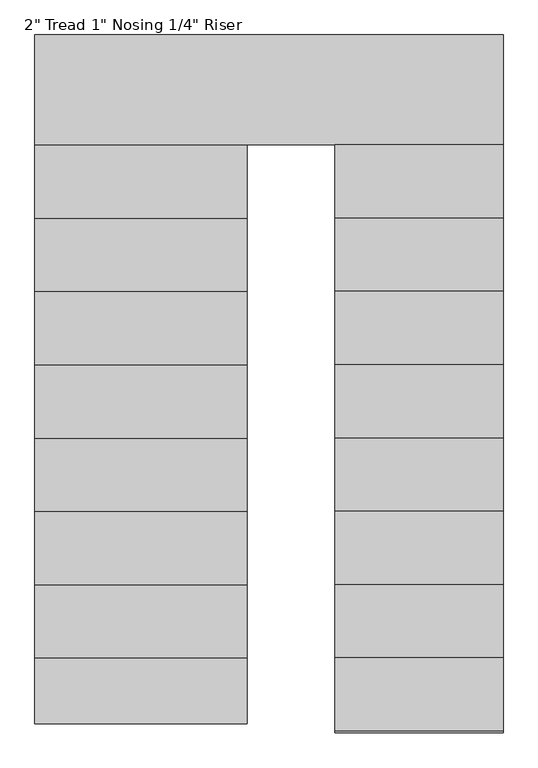
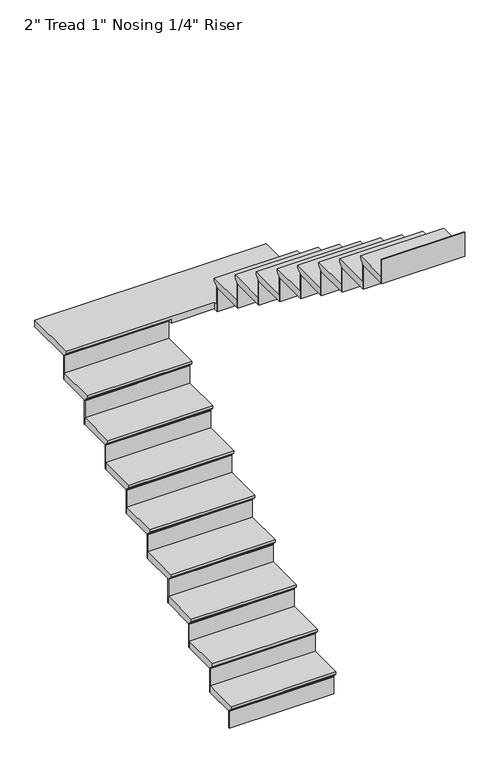
"""IFC4 building model written with IfcOpenShell, lengths in millimetres: stair flight geometry."""

from ifc_helpers import new_model, si_unit, origin, place, context, project, spatial, faceted_brep, source, transform, mapped, element, save


def stair_flight_4914edaa(model_context):
    return source(origin(), model_context, "Body", "Brep", [
        faceted_brep([(3394.0891134, -7650.9822004, 9759.95), (3394.0891134, -7650.9822004, 9779.0), (2657.4891134, -7650.9822004, 9779.0), (2657.4891134, -7650.9822004, 9759.95), (3394.0891134, -7625.5822004, 9734.55), (2657.4891134, -7625.5822004, 9734.55), (3394.0891134, -7396.9822004, 9779.0), (2657.4891134, -7396.9822004, 9779.0), (2657.4891134, -7625.5822004, 9728.2), (2657.4891134, -7396.9822004, 9728.2), (3394.0891134, -7396.9822004, 9728.2), (3394.0891134, -7625.5822004, 9728.2)], [[[0, 1, 2, 3]], [[4, 0, 3, 5]], [[2, 1, 6, 7]], [[8, 9, 10, 11]], [[2, 7, 9, 8, 5, 3]], [[8, 11, 4, 5]], [[6, 1, 0, 4, 11, 10]], [[7, 6, 10, 9]]]),
        faceted_brep([(3394.0891134, -7625.5822004, 9728.2), (3394.0891134, -7625.5822004, 9601.2), (3394.0891134, -7619.2322004, 9601.2), (3394.0891134, -7619.2322004, 9728.2), (2657.4891134, -7625.5822004, 9728.2), (2657.4891134, -7619.2322004, 9728.2), (2657.4891134, -7619.2322004, 9601.2), (2657.4891134, -7625.5822004, 9601.2)], [[[0, 1, 2, 3]], [[4, 5, 6, 7]], [[1, 0, 4, 7]], [[2, 1, 7, 6]], [[3, 2, 6, 5]], [[0, 3, 5, 4]]]),
        faceted_brep([(3394.0891134, -7396.9822004, 9906.0), (3394.0891134, -7396.9822004, 9728.2), (3394.0891134, -7390.6322004, 9728.2), (3394.0891134, -7390.6322004, 9906.0), (2657.4891134, -7396.9822004, 9906.0), (2657.4891134, -7390.6322004, 9906.0), (2657.4891134, -7390.6322004, 9728.2), (2657.4891134, -7396.9822004, 9728.2)], [[[0, 1, 2, 3]], [[4, 5, 6, 7]], [[1, 0, 4, 7]], [[2, 1, 7, 6]], [[3, 2, 6, 5]], [[0, 3, 5, 4]]]),
        faceted_brep([(2657.4891134, -7422.3822004, 9956.8), (3394.0891134, -7422.3822004, 9956.8), (3394.0891134, -7142.9822004, 9956.8), (2657.4891134, -7142.9822004, 9956.8), (2657.4891134, -7396.9822004, 9906.0), (2657.4891134, -7142.9822004, 9906.0), (3394.0891134, -7142.9822004, 9906.0), (3394.0891134, -7396.9822004, 9906.0), (2657.4891134, -7396.9822004, 9912.35), (2657.4891134, -7422.3822004, 9937.75), (3394.0891134, -7396.9822004, 9912.35), (3394.0891134, -7422.3822004, 9937.75)], [[[0, 1, 2, 3]], [[4, 5, 6, 7]], [[0, 3, 5, 4, 8, 9]], [[4, 7, 10, 8]], [[2, 1, 11, 10, 7, 6]], [[3, 2, 6, 5]], [[11, 1, 0, 9]], [[10, 11, 9, 8]]]),
        faceted_brep([(3394.0891134, -7142.9822004, 10083.8), (3394.0891134, -7142.9822004, 9906.0), (3394.0891134, -7136.6322004, 9906.0), (3394.0891134, -7136.6322004, 10083.8), (2657.4891134, -7142.9822004, 10083.8), (2657.4891134, -7136.6322004, 10083.8), (2657.4891134, -7136.6322004, 9906.0), (2657.4891134, -7142.9822004, 9906.0)], [[[0, 1, 2, 3]], [[4, 5, 6, 7]], [[1, 0, 4, 7]], [[2, 1, 7, 6]], [[3, 2, 6, 5]], [[0, 3, 5, 4]]]),
        faceted_brep([(2657.4891134, -7168.3822004, 10134.6), (3394.0891134, -7168.3822004, 10134.6), (3394.0891134, -6888.9822004, 10134.6), (2657.4891134, -6888.9822004, 10134.6), (2657.4891134, -7142.9822004, 10083.8), (2657.4891134, -6888.9822004, 10083.8), (3394.0891134, -6888.9822004, 10083.8), (3394.0891134, -7142.9822004, 10083.8), (2657.4891134, -7142.9822004, 10090.15), (2657.4891134, -7168.3822004, 10115.55), (3394.0891134, -7142.9822004, 10090.15), (3394.0891134, -7168.3822004, 10115.55)], [[[0, 1, 2, 3]], [[4, 5, 6, 7]], [[0, 3, 5, 4, 8, 9]], [[4, 7, 10, 8]], [[2, 1, 11, 10, 7, 6]], [[3, 2, 6, 5]], [[11, 1, 0, 9]], [[10, 11, 9, 8]]]),
        faceted_brep([(3394.0891134, -6888.9822004, 10261.6), (3394.0891134, -6888.9822004, 10083.8), (3394.0891134, -6882.6322004, 10083.8), (3394.0891134, -6882.6322004, 10261.6), (2657.4891134, -6888.9822004, 10261.6), (2657.4891134, -6882.6322004, 10261.6), (2657.4891134, -6882.6322004, 10083.8), (2657.4891134, -6888.9822004, 10083.8)], [[[0, 1, 2, 3]], [[4, 5, 6, 7]], [[1, 0, 4, 7]], [[2, 1, 7, 6]], [[3, 2, 6, 5]], [[0, 3, 5, 4]]]),
        faceted_brep([(2657.4891134, -6914.3822004, 10312.4), (3394.0891134, -6914.3822004, 10312.4), (3394.0891134, -6634.9822004, 10312.4), (2657.4891134, -6634.9822004, 10312.4), (2657.4891134, -6888.9822004, 10261.6), (2657.4891134, -6634.9822004, 10261.6), (3394.0891134, -6634.9822004, 10261.6), (3394.0891134, -6888.9822004, 10261.6), (2657.4891134, -6888.9822004, 10267.95), (2657.4891134, -6914.3822004, 10293.35), (3394.0891134, -6888.9822004, 10267.95), (3394.0891134, -6914.3822004, 10293.35)], [[[0, 1, 2, 3]], [[4, 5, 6, 7]], [[0, 3, 5, 4, 8, 9]], [[4, 7, 10, 8]], [[2, 1, 11, 10, 7, 6]], [[3, 2, 6, 5]], [[11, 1, 0, 9]], [[10, 11, 9, 8]]]),
        faceted_brep([(3394.0891134, -6634.9822004, 10439.4), (3394.0891134, -6634.9822004, 10261.6), (3394.0891134, -6628.6322004, 10261.6), (3394.0891134, -6628.6322004, 10439.4), (2657.4891134, -6634.9822004, 10439.4), (2657.4891134, -6628.6322004, 10439.4), (2657.4891134, -6628.6322004, 10261.6), (2657.4891134, -6634.9822004, 10261.6)], [[[0, 1, 2, 3]], [[4, 5, 6, 7]], [[1, 0, 4, 7]], [[2, 1, 7, 6]], [[3, 2, 6, 5]], [[0, 3, 5, 4]]]),
        faceted_brep([(2657.4891134, -6660.3822004, 10490.2), (3394.0891134, -6660.3822004, 10490.2), (3394.0891134, -6380.9822004, 10490.2), (2657.4891134, -6380.9822004, 10490.2), (2657.4891134, -6634.9822004, 10439.4), (2657.4891134, -6380.9822004, 10439.4), (3394.0891134, -6380.9822004, 10439.4), (3394.0891134, -6634.9822004, 10439.4), (2657.4891134, -6634.9822004, 10445.75), (2657.4891134, -6660.3822004, 10471.15), (3394.0891134, -6634.9822004, 10445.75), (3394.0891134, -6660.3822004, 10471.15)], [[[0, 1, 2, 3]], [[4, 5, 6, 7]], [[0, 3, 5, 4, 8, 9]], [[4, 7, 10, 8]], [[2, 1, 11, 10, 7, 6]], [[3, 2, 6, 5]], [[11, 1, 0, 9]], [[10, 11, 9, 8]]]),
        faceted_brep([(3394.0891134, -6380.9822004, 10617.2), (3394.0891134, -6380.9822004, 10439.4), (3394.0891134, -6374.6322004, 10439.4), (3394.0891134, -6374.6322004, 10617.2), (2657.4891134, -6380.9822004, 10617.2), (2657.4891134, -6374.6322004, 10617.2), (2657.4891134, -6374.6322004, 10439.4), (2657.4891134, -6380.9822004, 10439.4)], [[[0, 1, 2, 3]], [[4, 5, 6, 7]], [[1, 0, 4, 7]], [[2, 1, 7, 6]], [[3, 2, 6, 5]], [[0, 3, 5, 4]]]),
        faceted_brep([(2657.4891134, -6406.3822004, 10668.0), (3394.0891134, -6406.3822004, 10668.0), (3394.0891134, -6126.9822004, 10668.0), (2657.4891134, -6126.9822004, 10668.0), (2657.4891134, -6380.9822004, 10617.2), (2657.4891134, -6126.9822004, 10617.2), (3394.0891134, -6126.9822004, 10617.2), (3394.0891134, -6380.9822004, 10617.2), (2657.4891134, -6380.9822004, 10623.55), (2657.4891134, -6406.3822004, 10648.95), (3394.0891134, -6380.9822004, 10623.55), (3394.0891134, -6406.3822004, 10648.95)], [[[0, 1, 2, 3]], [[4, 5, 6, 7]], [[0, 3, 5, 4, 8, 9]], [[4, 7, 10, 8]], [[2, 1, 11, 10, 7, 6]], [[3, 2, 6, 5]], [[11, 1, 0, 9]], [[10, 11, 9, 8]]]),
        faceted_brep([(3394.0891134, -6126.9822004, 10795.0), (3394.0891134, -6126.9822004, 10617.2), (3394.0891134, -6120.6322004, 10617.2), (3394.0891134, -6120.6322004, 10795.0), (2657.4891134, -6126.9822004, 10795.0), (2657.4891134, -6120.6322004, 10795.0), (2657.4891134, -6120.6322004, 10617.2), (2657.4891134, -6126.9822004, 10617.2)], [[[0, 1, 2, 3]], [[4, 5, 6, 7]], [[1, 0, 4, 7]], [[2, 1, 7, 6]], [[3, 2, 6, 5]], [[0, 3, 5, 4]]]),
        faceted_brep([(2657.4891134, -6152.3822004, 10845.8), (3394.0891134, -6152.3822004, 10845.8), (3394.0891134, -5872.9822004, 10845.8), (2657.4891134, -5872.9822004, 10845.8), (2657.4891134, -6126.9822004, 10795.0), (2657.4891134, -5872.9822004, 10795.0), (3394.0891134, -5872.9822004, 10795.0), (3394.0891134, -6126.9822004, 10795.0), (2657.4891134, -6126.9822004, 10801.35), (2657.4891134, -6152.3822004, 10826.75), (3394.0891134, -6126.9822004, 10801.35), (3394.0891134, -6152.3822004, 10826.75)], [[[0, 1, 2, 3]], [[4, 5, 6, 7]], [[0, 3, 5, 4, 8, 9]], [[4, 7, 10, 8]], [[2, 1, 11, 10, 7, 6]], [[3, 2, 6, 5]], [[11, 1, 0, 9]], [[10, 11, 9, 8]]]),
        faceted_brep([(3394.0891134, -5872.9822004, 10972.8), (3394.0891134, -5872.9822004, 10795.0), (3394.0891134, -5866.6322004, 10795.0), (3394.0891134, -5866.6322004, 10972.8), (2657.4891134, -5872.9822004, 10972.8), (2657.4891134, -5866.6322004, 10972.8), (2657.4891134, -5866.6322004, 10795.0), (2657.4891134, -5872.9822004, 10795.0)], [[[0, 1, 2, 3]], [[4, 5, 6, 7]], [[1, 0, 4, 7]], [[2, 1, 7, 6]], [[3, 2, 6, 5]], [[0, 3, 5, 4]]]),
        faceted_brep([(2657.4891134, -5898.3822004, 11023.6), (3394.0891134, -5898.3822004, 11023.6), (3394.0891134, -5618.9822004, 11023.6), (2657.4891134, -5618.9822004, 11023.6), (2657.4891134, -5872.9822004, 10972.8), (2657.4891134, -5618.9822004, 10972.8), (3394.0891134, -5618.9822004, 10972.8), (3394.0891134, -5872.9822004, 10972.8), (2657.4891134, -5872.9822004, 10979.15), (2657.4891134, -5898.3822004, 11004.55), (3394.0891134, -5872.9822004, 10979.15), (3394.0891134, -5898.3822004, 11004.55)], [[[0, 1, 2, 3]], [[4, 5, 6, 7]], [[0, 3, 5, 4, 8, 9]], [[4, 7, 10, 8]], [[2, 1, 11, 10, 7, 6]], [[3, 2, 6, 5]], [[11, 1, 0, 9]], [[10, 11, 9, 8]]]),
        faceted_brep([(3394.0891134, -5618.9822004, 11150.6), (3394.0891134, -5618.9822004, 10972.8), (3394.0891134, -5612.6322004, 10972.8), (3394.0891134, -5612.6322004, 11150.6), (2657.4891134, -5618.9822004, 11150.6), (2657.4891134, -5612.6322004, 11150.6), (2657.4891134, -5612.6322004, 10972.8), (2657.4891134, -5618.9822004, 10972.8)], [[[0, 1, 2, 3]], [[4, 5, 6, 7]], [[1, 0, 4, 7]], [[2, 1, 7, 6]], [[3, 2, 6, 5]], [[0, 3, 5, 4]]]),
        faceted_brep([(4281.7311655, -5669.7822004, 11201.4), (4281.7311655, -5263.3822004, 11201.4), (2657.4891134, -5263.3822004, 11201.4), (2657.4891134, -5644.3822004, 11201.4), (3698.8891134, -5644.3822004, 11201.4), (3698.8891134, -5669.7822004, 11201.4), (4281.7311655, -5263.3822004, 11150.6), (4281.7311655, -5669.7822004, 11150.6), (3698.8891134, -5669.7822004, 11150.6), (3698.8891134, -5644.3822004, 11150.6), (3394.0891134, -5644.3822004, 11150.6), (3394.0891134, -5618.9822004, 11150.6), (2657.4891134, -5618.9822004, 11150.6), (2657.4891134, -5263.3822004, 11150.6), (3394.0891134, -5618.9822004, 11156.95), (2657.4891134, -5618.9822004, 11156.95), (2657.4891134, -5644.3822004, 11182.35), (3394.0891134, -5644.3822004, 11182.35)], [[[0, 1, 2, 3, 4, 5]], [[6, 7, 8, 9, 10, 11, 12, 13]], [[1, 0, 7, 6]], [[2, 1, 6, 13]], [[12, 11, 14, 15]], [[4, 3, 16, 17, 10, 9]], [[5, 4, 9, 8]], [[0, 5, 8, 7]], [[16, 15, 14, 17]], [[3, 2, 13, 12, 15, 16]], [[11, 10, 17, 14]]]),
        faceted_brep([(3698.8891134, -5669.7822004, 11328.4), (3698.8891134, -5669.7822004, 11150.6), (3698.8891134, -5676.1322004, 11150.6), (3698.8891134, -5676.1322004, 11328.4), (4281.7311655, -5669.7822004, 11328.4), (4281.7311655, -5676.1322004, 11328.4), (4281.7311655, -5676.1322004, 11150.6), (4281.7311655, -5669.7822004, 11150.6)], [[[0, 1, 2, 3]], [[4, 5, 6, 7]], [[1, 0, 4, 7]], [[2, 1, 7, 6]], [[3, 2, 6, 5]], [[0, 3, 5, 4]]]),
        faceted_brep([(4281.7311655, -5644.3822004, 11379.2), (3698.8891134, -5644.3822004, 11379.2), (3698.8891134, -5923.7822004, 11379.2), (4281.7311655, -5923.7822004, 11379.2), (4281.7311655, -5669.7822004, 11328.4), (4281.7311655, -5923.7822004, 11328.4), (3698.8891134, -5923.7822004, 11328.4), (3698.8891134, -5669.7822004, 11328.4), (4281.7311655, -5669.7822004, 11334.75), (4281.7311655, -5644.3822004, 11360.15), (3698.8891134, -5669.7822004, 11334.75), (3698.8891134, -5644.3822004, 11360.15)], [[[0, 1, 2, 3]], [[4, 5, 6, 7]], [[0, 3, 5, 4, 8, 9]], [[4, 7, 10, 8]], [[2, 1, 11, 10, 7, 6]], [[3, 2, 6, 5]], [[11, 1, 0, 9]], [[10, 11, 9, 8]]]),
        faceted_brep([(3698.8891134, -5923.7822004, 11506.2), (3698.8891134, -5923.7822004, 11328.4), (3698.8891134, -5930.1322004, 11328.4), (3698.8891134, -5930.1322004, 11506.2), (4281.7311655, -5923.7822004, 11506.2), (4281.7311655, -5930.1322004, 11506.2), (4281.7311655, -5930.1322004, 11328.4), (4281.7311655, -5923.7822004, 11328.4)], [[[0, 1, 2, 3]], [[4, 5, 6, 7]], [[1, 0, 4, 7]], [[2, 1, 7, 6]], [[3, 2, 6, 5]], [[0, 3, 5, 4]]]),
        faceted_brep([(4281.7311655, -5898.3822004, 11557.0), (3698.8891134, -5898.3822004, 11557.0), (3698.8891134, -6177.7822004, 11557.0), (4281.7311655, -6177.7822004, 11557.0), (4281.7311655, -5923.7822004, 11506.2), (4281.7311655, -6177.7822004, 11506.2), (3698.8891134, -6177.7822004, 11506.2), (3698.8891134, -5923.7822004, 11506.2), (4281.7311655, -5923.7822004, 11512.55), (4281.7311655, -5898.3822004, 11537.95), (3698.8891134, -5923.7822004, 11512.55), (3698.8891134, -5898.3822004, 11537.95)], [[[0, 1, 2, 3]], [[4, 5, 6, 7]], [[0, 3, 5, 4, 8, 9]], [[4, 7, 10, 8]], [[2, 1, 11, 10, 7, 6]], [[3, 2, 6, 5]], [[11, 1, 0, 9]], [[10, 11, 9, 8]]]),
        faceted_brep([(3698.8891134, -6177.7822004, 11684.0), (3698.8891134, -6177.7822004, 11506.2), (3698.8891134, -6184.1322004, 11506.2), (3698.8891134, -6184.1322004, 11684.0), (4281.7311655, -6177.7822004, 11684.0), (4281.7311655, -6184.1322004, 11684.0), (4281.7311655, -6184.1322004, 11506.2), (4281.7311655, -6177.7822004, 11506.2)], [[[0, 1, 2, 3]], [[4, 5, 6, 7]], [[1, 0, 4, 7]], [[2, 1, 7, 6]], [[3, 2, 6, 5]], [[0, 3, 5, 4]]]),
        faceted_brep([(4281.7311655, -6152.3822004, 11734.8), (3698.8891134, -6152.3822004, 11734.8), (3698.8891134, -6431.7822004, 11734.8), (4281.7311655, -6431.7822004, 11734.8), (4281.7311655, -6177.7822004, 11684.0), (4281.7311655, -6431.7822004, 11684.0), (3698.8891134, -6431.7822004, 11684.0), (3698.8891134, -6177.7822004, 11684.0), (4281.7311655, -6177.7822004, 11690.35), (4281.7311655, -6152.3822004, 11715.75), (3698.8891134, -6177.7822004, 11690.35), (3698.8891134, -6152.3822004, 11715.75)], [[[0, 1, 2, 3]], [[4, 5, 6, 7]], [[0, 3, 5, 4, 8, 9]], [[4, 7, 10, 8]], [[2, 1, 11, 10, 7, 6]], [[3, 2, 6, 5]], [[11, 1, 0, 9]], [[10, 11, 9, 8]]]),
        faceted_brep([(3698.8891134, -6431.7822004, 11861.8), (3698.8891134, -6431.7822004, 11684.0), (3698.8891134, -6438.1322004, 11684.0), (3698.8891134, -6438.1322004, 11861.8), (4281.7311655, -6431.7822004, 11861.8), (4281.7311655, -6438.1322004, 11861.8), (4281.7311655, -6438.1322004, 11684.0), (4281.7311655, -6431.7822004, 11684.0)], [[[0, 1, 2, 3]], [[4, 5, 6, 7]], [[1, 0, 4, 7]], [[2, 1, 7, 6]], [[3, 2, 6, 5]], [[0, 3, 5, 4]]]),
        faceted_brep([(4281.7311655, -6406.3822004, 11912.6), (3698.8891134, -6406.3822004, 11912.6), (3698.8891134, -6685.7822004, 11912.6), (4281.7311655, -6685.7822004, 11912.6), (4281.7311655, -6431.7822004, 11861.8), (4281.7311655, -6685.7822004, 11861.8), (3698.8891134, -6685.7822004, 11861.8), (3698.8891134, -6431.7822004, 11861.8), (4281.7311655, -6431.7822004, 11868.15), (4281.7311655, -6406.3822004, 11893.55), (3698.8891134, -6431.7822004, 11868.15), (3698.8891134, -6406.3822004, 11893.55)], [[[0, 1, 2, 3]], [[4, 5, 6, 7]], [[0, 3, 5, 4, 8, 9]], [[4, 7, 10, 8]], [[2, 1, 11, 10, 7, 6]], [[3, 2, 6, 5]], [[11, 1, 0, 9]], [[10, 11, 9, 8]]]),
        faceted_brep([(3698.8891134, -6685.7822004, 12039.6), (3698.8891134, -6685.7822004, 11861.8), (3698.8891134, -6692.1322004, 11861.8), (3698.8891134, -6692.1322004, 12039.6), (4281.7311655, -6685.7822004, 12039.6), (4281.7311655, -6692.1322004, 12039.6), (4281.7311655, -6692.1322004, 11861.8), (4281.7311655, -6685.7822004, 11861.8)], [[[0, 1, 2, 3]], [[4, 5, 6, 7]], [[1, 0, 4, 7]], [[2, 1, 7, 6]], [[3, 2, 6, 5]], [[0, 3, 5, 4]]]),
        faceted_brep([(4281.7311655, -6660.3822004, 12090.4), (3698.8891134, -6660.3822004, 12090.4), (3698.8891134, -6939.7822004, 12090.4), (4281.7311655, -6939.7822004, 12090.4), (4281.7311655, -6685.7822004, 12039.6), (4281.7311655, -6939.7822004, 12039.6), (3698.8891134, -6939.7822004, 12039.6), (3698.8891134, -6685.7822004, 12039.6), (4281.7311655, -6685.7822004, 12045.95), (4281.7311655, -6660.3822004, 12071.35), (3698.8891134, -6685.7822004, 12045.95), (3698.8891134, -6660.3822004, 12071.35)], [[[0, 1, 2, 3]], [[4, 5, 6, 7]], [[0, 3, 5, 4, 8, 9]], [[4, 7, 10, 8]], [[2, 1, 11, 10, 7, 6]], [[3, 2, 6, 5]], [[11, 1, 0, 9]], [[10, 11, 9, 8]]]),
        faceted_brep([(3698.8891134, -6939.7822004, 12217.4), (3698.8891134, -6939.7822004, 12039.6), (3698.8891134, -6946.1322004, 12039.6), (3698.8891134, -6946.1322004, 12217.4), (4281.7311655, -6939.7822004, 12217.4), (4281.7311655, -6946.1322004, 12217.4), (4281.7311655, -6946.1322004, 12039.6), (4281.7311655, -6939.7822004, 12039.6)], [[[0, 1, 2, 3]], [[4, 5, 6, 7]], [[1, 0, 4, 7]], [[2, 1, 7, 6]], [[3, 2, 6, 5]], [[0, 3, 5, 4]]]),
        faceted_brep([(4281.7311655, -6914.3822004, 12268.2), (3698.8891134, -6914.3822004, 12268.2), (3698.8891134, -7193.7822004, 12268.2), (4281.7311655, -7193.7822004, 12268.2), (4281.7311655, -6939.7822004, 12217.4), (4281.7311655, -7193.7822004, 12217.4), (3698.8891134, -7193.7822004, 12217.4), (3698.8891134, -6939.7822004, 12217.4), (4281.7311655, -6939.7822004, 12223.75), (4281.7311655, -6914.3822004, 12249.15), (3698.8891134, -6939.7822004, 12223.75), (3698.8891134, -6914.3822004, 12249.15)], [[[0, 1, 2, 3]], [[4, 5, 6, 7]], [[0, 3, 5, 4, 8, 9]], [[4, 7, 10, 8]], [[2, 1, 11, 10, 7, 6]], [[3, 2, 6, 5]], [[11, 1, 0, 9]], [[10, 11, 9, 8]]]),
        faceted_brep([(3698.8891134, -7193.7822004, 12395.2), (3698.8891134, -7193.7822004, 12217.4), (3698.8891134, -7200.1322004, 12217.4), (3698.8891134, -7200.1322004, 12395.2), (4281.7311655, -7193.7822004, 12395.2), (4281.7311655, -7200.1322004, 12395.2), (4281.7311655, -7200.1322004, 12217.4), (4281.7311655, -7193.7822004, 12217.4)], [[[0, 1, 2, 3]], [[4, 5, 6, 7]], [[1, 0, 4, 7]], [[2, 1, 7, 6]], [[3, 2, 6, 5]], [[0, 3, 5, 4]]]),
        faceted_brep([(4281.7311655, -7168.3822004, 12446.0), (3698.8891134, -7168.3822004, 12446.0), (3698.8891134, -7447.7822004, 12446.0), (4281.7311655, -7447.7822004, 12446.0), (4281.7311655, -7193.7822004, 12395.2), (4281.7311655, -7447.7822004, 12395.2), (3698.8891134, -7447.7822004, 12395.2), (3698.8891134, -7193.7822004, 12395.2), (4281.7311655, -7193.7822004, 12401.55), (4281.7311655, -7168.3822004, 12426.95), (3698.8891134, -7193.7822004, 12401.55), (3698.8891134, -7168.3822004, 12426.95)], [[[0, 1, 2, 3]], [[4, 5, 6, 7]], [[0, 3, 5, 4, 8, 9]], [[4, 7, 10, 8]], [[2, 1, 11, 10, 7, 6]], [[3, 2, 6, 5]], [[11, 1, 0, 9]], [[10, 11, 9, 8]]]),
        faceted_brep([(3698.8891134, -7447.7822004, 12573.0), (3698.8891134, -7447.7822004, 12395.2), (3698.8891134, -7454.1322004, 12395.2), (3698.8891134, -7454.1322004, 12573.0), (4281.7311655, -7447.7822004, 12573.0), (4281.7311655, -7454.1322004, 12573.0), (4281.7311655, -7454.1322004, 12395.2), (4281.7311655, -7447.7822004, 12395.2)], [[[0, 1, 2, 3]], [[4, 5, 6, 7]], [[1, 0, 4, 7]], [[2, 1, 7, 6]], [[3, 2, 6, 5]], [[0, 3, 5, 4]]]),
        faceted_brep([(3698.8891134, -7676.3822004, 12750.8), (3698.8891134, -7676.3822004, 12573.0), (3698.8891134, -7682.7322004, 12573.0), (3698.8891134, -7682.7322004, 12750.8), (4281.7311655, -7676.3822004, 12750.8), (4281.7311655, -7682.7322004, 12750.8), (4281.7311655, -7682.7322004, 12573.0), (4281.7311655, -7676.3822004, 12573.0)], [[[0, 1, 2, 3]], [[4, 5, 6, 7]], [[1, 0, 4, 7]], [[2, 1, 7, 6]], [[3, 2, 6, 5]], [[0, 3, 5, 4]]]),
        faceted_brep([(4281.7311655, -7422.3822004, 12623.8), (3698.8891134, -7422.3822004, 12623.8), (3698.8891134, -7676.3822004, 12623.8), (4281.7311655, -7676.3822004, 12623.8), (4281.7311655, -7447.7822004, 12573.0), (4281.7311655, -7676.3822004, 12573.0), (3698.8891134, -7676.3822004, 12573.0), (3698.8891134, -7447.7822004, 12573.0), (4281.7311655, -7447.7822004, 12579.35), (4281.7311655, -7422.3822004, 12604.75), (3698.8891134, -7447.7822004, 12579.35), (3698.8891134, -7422.3822004, 12604.75)], [[[0, 1, 2, 3]], [[4, 5, 6, 7]], [[0, 3, 5, 4, 8, 9]], [[4, 7, 10, 8]], [[2, 1, 11, 10, 7, 6]], [[3, 2, 6, 5]], [[11, 1, 0, 9]], [[10, 11, 9, 8]]]),
    ])


if __name__ == "__main__":
    model = new_model("IFC4")
    model_context = context("Model", 3, world=origin())
    ifc_project = project(units=[si_unit("LENGTHUNIT", "METRE", prefix="MILLI")], contexts=[model_context])
    site = spatial("IfcSite", under=ifc_project)
    building = spatial("IfcBuilding", under=site)
    placement = place(None, origin())
    stair_flight_shape = stair_flight_4914edaa(model_context)
    element("IfcStairFlight", 1, ObjectType="2\" Tread 1\" Nosing 1/4\" Riser", at=placement, inside=building, context=model_context, shape_type="MappedRepresentation", body=[
        mapped(stair_flight_shape, transform((0.0, 0.0, 0.0), x_axis=(1.0, 0.0, 0.0), y_axis=(0.0, 1.0, 0.0), z_axis=(0.0, 0.0, 1.0))),
    ])
    save(model, "model.ifc")
